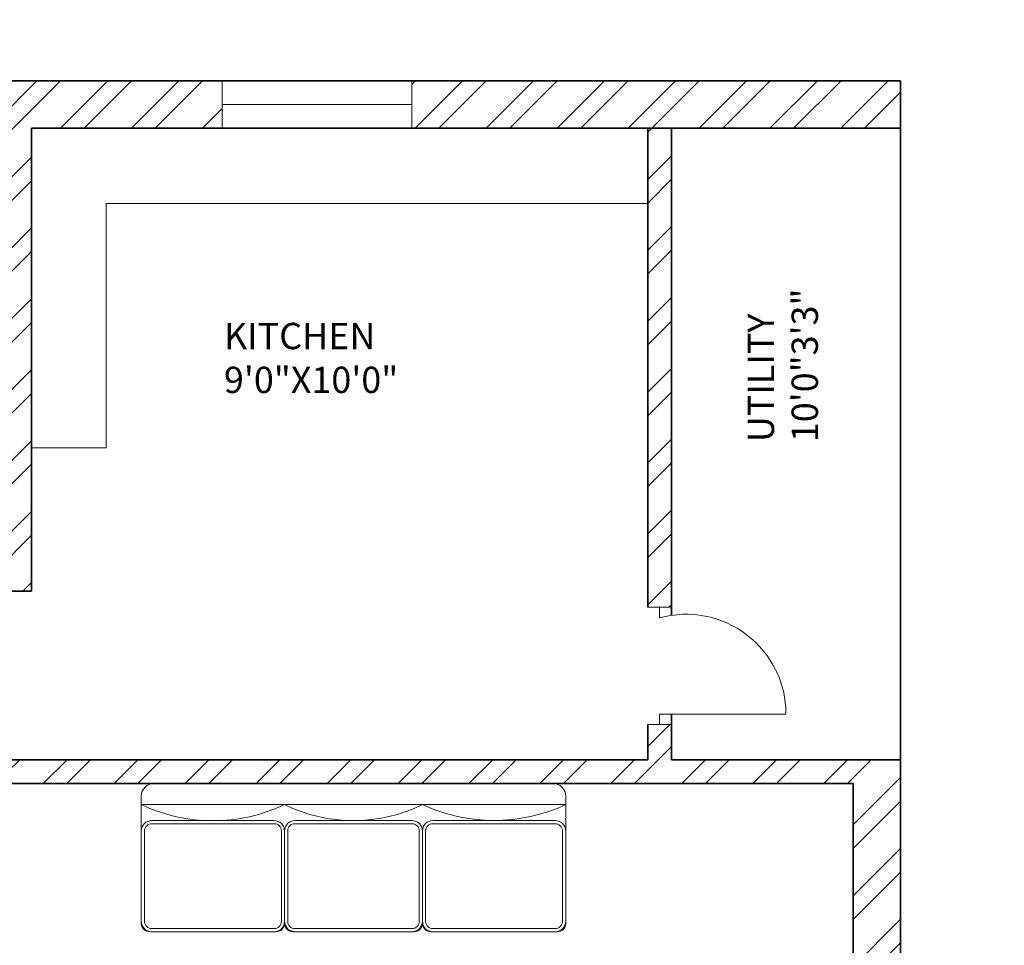
# Model space of a CAD drawing. Units: inches. Extents: x 2120 to 4013, y 1390 to 3019.
# Tile 34 of 59: x 2470 to 2657, y 2188 to 2364. Entities that reach past the tile are written whole.
import ezdxf

# ---------------------------------------------------------------- set-up
doc = ezdxf.new("R2010")
doc.units = ezdxf.units.IN
for name, color, linetype, lineweight in [('A-ANNO-DIMS', 2, 'Continuous', 18), ('A-AREA-IDEN', 7, 'Continuous', 18), ('A-DOOR', 3, 'Continuous', 18), ('A-FLOR-CASE', 8, 'Continuous', 18), ('A-FURN', 8, 'Continuous', 13), ('A-GLAZ', 4, 'Continuous', 18), ('A-WALL', 7, 'Continuous', 35), ('A-WALL-PATT', 252, 'Continuous', 13)]:
    doc.layers.add(name, color=color, linetype=linetype, lineweight=lineweight)
doc.styles.get("Standard").update_dxf_attribs({"font": 'arial.ttf'})
doc.dimstyles.get("Standard").update_dxf_attribs({"dimtxt": 0.18, "dimasz": 0.18, "dimexe": 0.18, "dimexo": 0.0625, "dimgap": 0.09, "dimtad": 0, "dimtih": 1, "dimtoh": 1, "dimdec": 4, "dimzin": 0, "dimdsep": 46, "dimtxsty": 'Standard', "dimcen": 0.09, "dimadec": 0, "dimazin": 0, "dimtfac": 1, "dimtdec": 4, "dimtofl": 0, "dimtmove": 0, "dimatfit": 3, "dimfxl": 1, "dimtolj": 1, "dimtzin": 0, "dimarcsym": 0})

# ---------------------------------------------------------------- blocks, each defined once
blk = doc.blocks.new('DOOR-SWING-24IN-105p37DEG')
for p, q in [((4.5, 22.29), (0, 22.29)), ((0, 22.29), (2.25, 22.29)), ((2.25, 22.29), (2.25, 20.29)), ((2.25, 0), (2.25, 2)), ((2.25, 2), (26.25, 2)), ((0, 0), (4.5, 0)), ((4.5, 0), (2.25, 0))]:
    blk.add_line(p, q)
blk.add_arc((7.28, 2), 18.97, 0, 105.3718)
blk = doc.blocks.new('WIN-PLAN-36IN')
for p, q in [((0, 0), (0, 9)), ((0, 9), (0, 4.5)), ((36, 4.5), (36, 9)), ((36, 9), (36, 0)), ((0, 4.5), (36, 4.5))]:
    blk.add_line(p, q)
blk = doc.blocks.new('*D211')
at = {"layer": 'A-ANNO-DIMS', "color": 0, "lineweight": -2, "transparency": 16777216}
for p, q in [((2262.73, 2352.59), (2262.73, 2397.71)), ((2262.91, 2397.53), (2635.95, 2397.53)), ((3009.55, 2397.53), (2636.52, 2397.53)), ((3009.73, 2352.59), (3009.73, 2397.71))]:
    blk.add_line(p, q, dxfattribs=at)
at = {"layer": 'A-ANNO-DIMS', "color": 0, "transparency": 16777216}
for points in [[(2262.91, 2397.56), (2262.91, 2397.5), (2262.73, 2397.53)], [(3009.55, 2397.56), (3009.55, 2397.5), (3009.73, 2397.53)]]:
    blk.add_solid(points, dxfattribs=at)
at = {"layer": 'Defpoints', "color": 0, "transparency": 16777216}
for p in [(3009.73, 2397.53), (2262.73, 2352.53), (3009.73, 2352.53)]:
    blk.add_point(p, dxfattribs=at)
at = {"layer": 'A-ANNO-DIMS', "color": 0, "transparency": 16777216, "insert": (2636.23, 2397.53), "char_height": 0.18, "attachment_point": 5}
blk.add_mtext('\\A1;747', dxfattribs=at)

msp = doc.modelspace()

# ---------------------------------------------------------------- hatches: boundary and pattern name
at = {"layer": 'A-WALL-PATT'}
h = msp.add_hatch(dxfattribs=at)
h.set_pattern_fill('ANSI32', color=256)
h.paths.add_polyline_path([(2271.7331, 2343.531), (2283.3788, 2343.531), (2283.3788, 2348.031), (2283.3788, 2352.5306), (2262.7331, 2352.5306), (2262.7331, 2182.638), (2267.2331, 2182.638), (2271.7331, 2182.638), (2271.7331, 2219.031), (2391.7331, 2219.031), (2391.7331, 2214.189), (2393.9831, 2214.189), (2396.2331, 2214.189), (2396.2331, 2219.031), (2420.2331, 2219.031), (2420.2331, 2225.7535), (2417.2197, 2225.7535), (2415.7331, 2225.7535), (2415.7331, 2223.5306), (2271.7331, 2223.5306)])
h.paths.add_polyline_path([(2380.0942, 2352.5306), (2343.3788, 2352.5306), (2343.3788, 2343.531), (2363.2331, 2343.531), (2363.2331, 2288.8489), (2365.4831, 2288.8489), (2367.7331, 2288.8489), (2367.7331, 2343.531), (2380.0942, 2343.531)], flags=17)
h.paths.add_polyline_path([(2432.4339, 2352.5306), (2404.0943, 2352.5306), (2404.0943, 2343.531), (2415.7331, 2343.531), (2415.7331, 2264.0306), (2367.7331, 2264.0306), (2367.7331, 2266.4872), (2363.2331, 2266.4872), (2363.2331, 2259.531), (2367.7331, 2259.531), (2415.7331, 2259.531), (2415.7331, 2255.0658), (2420.2331, 2255.0658), (2420.2331, 2259.531), (2424.5717, 2259.531), (2424.5717, 2261.781), (2424.5717, 2264.0306), (2420.2331, 2264.0306), (2420.2331, 2343.531), (2432.4339, 2343.531)])
h.paths.add_polyline_path([(2508.9115, 2352.5306), (2456.4339, 2352.5306), (2456.4339, 2343.531), (2468.2331, 2343.531), (2468.2331, 2264.0306), (2448.0487, 2264.0306), (2448.0487, 2259.531), (2468.2331, 2259.531), (2468.2331, 2255.5496), (2472.7331, 2255.5496), (2472.7331, 2343.531), (2508.9115, 2343.531)])
h.paths.add_polyline_path([(2637.7331, 2352.5306), (2544.9116, 2352.5306), (2544.9116, 2343.531), (2589.7331, 2343.531), (2633.2331, 2343.531), (2637.7331, 2343.531)])
h.paths.add_polyline_path([(2594.2331, 2343.5306), (2589.7331, 2343.5306), (2589.7331, 2259.5306), (2589.7331, 2252.4915), (2591.9831, 2252.4915), (2594.2331, 2252.4915)])
h.paths.add_polyline_path([(2637.7331, 2223.5306), (2594.2331, 2223.5306), (2594.2331, 2230.1988), (2591.9831, 2230.1988), (2589.7331, 2230.1988), (2589.7331, 2223.5306), (2472.7331, 2223.5306), (2468.2331, 2223.5306), (2468.2331, 2219.031), (2628.7331, 2219.031), (2628.7331, 2138.031), (2637.7331, 2138.031)])
h.paths.add_polyline_path([(3822.6535, 2458.4402), (3874.9468, 2458.4402), (3874.9468, 2476.9866), (3822.6535, 2476.9866)], flags=9)
h.paths.add_polyline_path([(3834.6921, 2781.8174), (3935.9206, 2781.8174), (3935.9206, 2800.3638), (3834.6921, 2800.3638)], flags=9)
h.paths.add_polyline_path([(3832.2843, 2837.9683), (3884.5776, 2837.9683), (3884.5776, 2856.5146), (3832.2843, 2856.5146)], flags=9)
h.paths.add_polyline_path([(3830.9388, 2861.4782), (3956.8958, 2861.4782), (3956.8958, 2880.0245), (3830.9388, 2880.0245)], flags=9)
h.paths.add_polyline_path([(3870.6966, 2352.5752), (3887.9272, 2352.5752), (3887.9272, 2377.3037), (3870.6966, 2377.3037)], flags=9)
h.paths.add_polyline_path([(3289.2701, 2413.161), (3435.2223, 2413.161), (3435.2223, 2450.2538), (3289.2701, 2450.2538)], flags=9)
h.paths.add_polyline_path([(2487.6944, 2414.3601), (2637.8335, 2414.3601), (2637.8335, 2451.4528), (2487.6944, 2451.4528)], flags=9)
h.paths.add_polyline_path([(2567.3724, 1457.9199), (2815.296, 1457.9199), (2815.296, 1495.0127), (2567.3724, 1495.0127)], flags=9)
h.paths.add_polyline_path([(2655.3825, 2093.2363), (2685.9555, 2093.2363), (2685.9555, 2111.8937), (2655.3825, 2111.8937)], flags=9)
h.paths.add_polyline_path([(2543.9218, 1550.6671), (2587.8406, 1550.6671), (2587.8406, 1569.3244), (2543.9218, 1569.3244)], flags=9)
h.paths.add_polyline_path([(2905.1384, 1543.8113), (2949.0572, 1543.8113), (2949.0572, 1562.4686), (2905.1384, 1562.4686)], flags=9)
h.paths.add_polyline_path([(2736.4118, 1702.4736), (2784.2153, 1702.4736), (2784.2153, 1721.1309), (2736.4118, 1721.1309)], flags=9)
h.paths.add_polyline_path([(2912.8666, 1710.4168), (2951.707, 1710.4168), (2951.707, 1729.0741), (2912.8666, 1729.0741)], flags=9)
h.paths.add_polyline_path([(2923.5785, 1763.5038), (2959.7279, 1763.5038), (2959.7279, 1782.1611), (2923.5785, 1782.1611)], flags=9)
h.paths.add_polyline_path([(2925.2114, 1809.6137), (2967.1861, 1809.6137), (2967.1861, 1828.271), (2925.2114, 1828.271)], flags=9)
h.paths.add_polyline_path([(2996.2711, 1878.9003), (2996.2711, 1913.109), (2977.6138, 1913.109), (2977.6138, 1878.9003)], flags=9)
h.paths.add_polyline_path([(2883.0859, 1895.7192), (2927.1855, 1895.7192), (2927.1855, 1914.3766), (2883.0859, 1914.3766)], flags=9)
h.paths.add_polyline_path([(2787.3924, 1810.8013), (2841.0213, 1810.8013), (2841.0213, 1829.4587), (2787.3924, 1829.4587)], flags=9)
h.paths.add_polyline_path([(2775.6399, 2101.7395), (2829.2689, 2101.7395), (2829.2689, 2120.3968), (2775.6399, 2120.3968)], flags=9)
h.paths.add_polyline_path([(2913.0263, 2075.817), (2951.8667, 2075.817), (2951.8667, 2094.4744), (2913.0263, 2094.4744)], flags=9)
h.paths.add_polyline_path([(2929.966, 2133.3669), (2966.1154, 2133.3669), (2966.1154, 2152.0243), (2929.966, 2152.0243)], flags=9)
h.paths.add_polyline_path([(2932.7502, 2182.6088), (2968.8996, 2182.6088), (2968.8996, 2201.2662), (2932.7502, 2201.2662)], flags=9)
h.paths.add_polyline_path([(2996.0681, 2266.3173), (2996.0681, 2300.5261), (2977.4108, 2300.5261), (2977.4108, 2266.3173)], flags=9)
h.paths.add_polyline_path([(2885.1039, 2279.2186), (2929.2035, 2279.2186), (2929.2035, 2297.8759), (2885.1039, 2297.8759)], flags=9)
h.paths.add_polyline_path([(2735.7042, 2218.3197), (2783.5078, 2218.3197), (2783.5078, 2236.9771), (2735.7042, 2236.9771)], flags=9)
h.paths.add_polyline_path([(2635.6049, 2044.0085), (2648.9678, 2044.0085), (2648.9678, 2054.312), (2635.6049, 2054.312)], flags=9)
h.paths.add_polyline_path([(2714.0148, 1923.0473), (2727.3777, 1923.0473), (2727.3777, 1933.3508), (2714.0148, 1933.3508)], flags=9)
h.paths.add_polyline_path([(2709.0345, 1988.1628), (2722.3974, 1988.1628), (2722.3974, 1998.4663), (2709.0345, 1998.4663)], flags=9)
h.paths.add_polyline_path([(2592.8935, 1962.1763), (2606.2564, 1962.1763), (2606.2564, 1972.4799), (2592.8935, 1972.4799)], flags=9)
h.paths.add_polyline_path([(2618.3996, 1985.9724), (2644.1942, 1985.9724), (2644.1942, 1996.2759), (2618.3996, 1996.2759)], flags=9)
h.paths.add_polyline_path([(2601.279, 1920.5869), (2614.6419, 1920.5869), (2614.6419, 1930.8904), (2601.279, 1930.8904)], flags=9)
h.paths.add_polyline_path([(2692.3278, 1932.7645), (2704.5311, 1932.7645), (2704.5311, 1943.0681), (2692.3278, 1943.0681)], flags=9)
h.paths.add_polyline_path([(2311.122, 1672.7318), (2355.0408, 1672.7318), (2355.0408, 1691.3892), (2311.122, 1691.3892)], flags=9)
h.paths.add_polyline_path([(2456.2551, 1632.3198), (2492.4796, 1632.3198), (2492.4796, 1650.9772), (2456.2551, 1650.9772)], flags=9)
h.paths.add_polyline_path([(2401.0766, 1631.4793), (2437.301, 1631.4793), (2437.301, 1650.1367), (2401.0766, 1650.1367)], flags=9)
h.paths.add_polyline_path([(2546.7054, 1700.9235), (2594.509, 1700.9235), (2594.509, 1719.5809), (2546.7054, 1719.5809)], flags=9)
h.paths.add_polyline_path([(2445.4866, 1766.9937), (2497.5261, 1766.9937), (2497.5261, 1785.651), (2445.4866, 1785.651)], flags=9)
h.paths.add_polyline_path([(2287.9992, 1739.7675), (2326.8396, 1739.7675), (2326.8396, 1758.4248), (2287.9992, 1758.4248)], flags=9)
h.paths.add_polyline_path([(2458.5279, 1924.7607), (2510.5675, 1924.7607), (2510.5675, 1943.4181), (2458.5279, 1943.4181)], flags=9)
h.paths.add_polyline_path([(2309.2811, 1902.7642), (2345.4305, 1902.7642), (2345.4305, 1921.4215), (2309.2811, 1921.4215)], flags=9)
h.paths.add_polyline_path([(2490.7554, 2018.9392), (2530.7896, 2018.9392), (2530.7896, 2037.5965), (2490.7554, 2037.5965)], flags=9)
h.paths.add_polyline_path([(2402.143, 2024.7393), (2438.5414, 2024.7393), (2438.5414, 2043.3966), (2402.143, 2043.3966)], flags=9)
h.paths.add_polyline_path([(2287.856, 1931.7926), (2326.6964, 1931.7926), (2326.6964, 1950.4499), (2287.856, 1950.4499)], flags=9)
h.paths.add_polyline_path([(2281.7979, 2193.5771), (2320.6383, 2193.5771), (2320.6383, 2212.2344), (2281.7979, 2212.2344)], flags=25)
h.paths.add_polyline_path([(2484.0754, 2093.892), (2536.115, 2093.892), (2536.115, 2112.5494), (2484.0754, 2112.5494)], flags=9)
h.paths.add_polyline_path([(2624.7948, 2281.8639), (2624.7948, 2311.4137), (2606.1375, 2311.4137), (2606.1375, 2281.8639)], flags=9)
h.paths.add_polyline_path([(2507.5036, 2290.3639), (2541.934, 2290.3639), (2541.934, 2309.0212), (2507.5036, 2309.0212)], flags=9)
h.paths.add_polyline_path([(2423.1076, 2285.2202), (2459.332, 2285.2202), (2459.332, 2303.8776), (2423.1076, 2303.8776)], flags=9)
h.paths.add_polyline_path([(2374.5467, 2289.6272), (2410.7711, 2289.6272), (2410.7711, 2308.2846), (2374.5467, 2308.2846)], flags=25)
h.paths.add_polyline_path([(2277.4907, 2227.5651), (2316.3311, 2227.5651), (2316.3311, 2246.2224), (2277.4907, 2246.2224)], flags=25)
h.paths.add_polyline_path([(2655.3825, 2093.2367), (2685.9555, 2093.2367), (2685.9555, 2111.894), (2655.3825, 2111.894)], flags=9)
h.paths.add_polyline_path([(2543.9217, 1550.6674), (2587.8406, 1550.6674), (2587.8406, 1569.3247), (2543.9217, 1569.3247)], flags=9)
h.paths.add_polyline_path([(2905.1384, 1543.8116), (2949.0572, 1543.8116), (2949.0572, 1562.4689), (2905.1384, 1562.4689)], flags=9)
h.paths.add_polyline_path([(2736.4118, 1702.4739), (2784.2153, 1702.4739), (2784.2153, 1721.1312), (2736.4118, 1721.1312)], flags=9)
h.paths.add_polyline_path([(2912.8666, 1710.4171), (2951.707, 1710.4171), (2951.707, 1729.0744), (2912.8666, 1729.0744)], flags=9)
h.paths.add_polyline_path([(2923.5785, 1763.5041), (2959.7279, 1763.5041), (2959.7279, 1782.1614), (2923.5785, 1782.1614)], flags=9)
h.paths.add_polyline_path([(2925.2114, 1809.614), (2967.1861, 1809.614), (2967.1861, 1828.2713), (2925.2114, 1828.2713)], flags=9)
h.paths.add_polyline_path([(2996.2711, 1878.9006), (2996.2711, 1913.1094), (2977.6137, 1913.1094), (2977.6137, 1878.9006)], flags=9)
h.paths.add_polyline_path([(2883.0859, 1895.7195), (2927.1855, 1895.7195), (2927.1855, 1914.3769), (2883.0859, 1914.3769)], flags=9)
h.paths.add_polyline_path([(2787.3924, 1810.8016), (2841.0213, 1810.8016), (2841.0213, 1829.459), (2787.3924, 1829.459)], flags=9)
h.paths.add_polyline_path([(2775.6399, 2101.7398), (2829.2688, 2101.7398), (2829.2688, 2120.3971), (2775.6399, 2120.3971)], flags=9)
h.paths.add_polyline_path([(2913.0263, 2075.8173), (2951.8667, 2075.8173), (2951.8667, 2094.4747), (2913.0263, 2094.4747)], flags=9)
h.paths.add_polyline_path([(2929.966, 2133.3672), (2966.1154, 2133.3672), (2966.1154, 2152.0246), (2929.966, 2152.0246)], flags=9)
h.paths.add_polyline_path([(2932.7502, 2182.6091), (2968.8996, 2182.6091), (2968.8996, 2201.2665), (2932.7502, 2201.2665)], flags=9)
h.paths.add_polyline_path([(2996.0681, 2266.3176), (2996.0681, 2300.5264), (2977.4108, 2300.5264), (2977.4108, 2266.3176)], flags=9)
h.paths.add_polyline_path([(2885.1039, 2279.2189), (2929.2035, 2279.2189), (2929.2035, 2297.8762), (2885.1039, 2297.8762)], flags=9)
h.paths.add_polyline_path([(2735.7042, 2218.32), (2783.5078, 2218.32), (2783.5078, 2236.9774), (2735.7042, 2236.9774)], flags=9)
h.paths.add_polyline_path([(2635.6048, 2044.0088), (2648.9677, 2044.0088), (2648.9677, 2054.3123), (2635.6048, 2054.3123)], flags=9)
h.paths.add_polyline_path([(2714.0148, 1923.0476), (2727.3777, 1923.0476), (2727.3777, 1933.3511), (2714.0148, 1933.3511)], flags=9)
h.paths.add_polyline_path([(2709.0345, 1988.1631), (2722.3974, 1988.1631), (2722.3974, 1998.4666), (2709.0345, 1998.4666)], flags=9)
h.paths.add_polyline_path([(2592.8935, 1962.1766), (2606.2564, 1962.1766), (2606.2564, 1972.4802), (2592.8935, 1972.4802)], flags=9)
h.paths.add_polyline_path([(2618.3995, 1985.9727), (2644.1942, 1985.9727), (2644.1942, 1996.2762), (2618.3995, 1996.2762)], flags=9)
h.paths.add_polyline_path([(2601.279, 1920.5872), (2614.6419, 1920.5872), (2614.6419, 1930.8908), (2601.279, 1930.8908)], flags=9)
h.paths.add_polyline_path([(2692.3278, 1932.7648), (2704.5311, 1932.7648), (2704.5311, 1943.0684), (2692.3278, 1943.0684)], flags=9)
h.paths.add_polyline_path([(2311.122, 1672.7321), (2355.0408, 1672.7321), (2355.0408, 1691.3895), (2311.122, 1691.3895)], flags=9)
h.paths.add_polyline_path([(2456.2551, 1632.3201), (2492.4795, 1632.3201), (2492.4795, 1650.9775), (2456.2551, 1650.9775)], flags=9)
h.paths.add_polyline_path([(2401.0766, 1631.4796), (2437.301, 1631.4796), (2437.301, 1650.137), (2401.0766, 1650.137)], flags=9)
h.paths.add_polyline_path([(2546.7054, 1700.9238), (2594.509, 1700.9238), (2594.509, 1719.5812), (2546.7054, 1719.5812)], flags=9)
h.paths.add_polyline_path([(2445.4866, 1766.994), (2497.5261, 1766.994), (2497.5261, 1785.6513), (2445.4866, 1785.6513)], flags=9)
h.paths.add_polyline_path([(2287.9992, 1739.7678), (2326.8396, 1739.7678), (2326.8396, 1758.4251), (2287.9992, 1758.4251)], flags=9)
h.paths.add_polyline_path([(2458.5279, 1924.7611), (2510.5675, 1924.7611), (2510.5675, 1943.4184), (2458.5279, 1943.4184)], flags=9)
h.paths.add_polyline_path([(2309.2811, 1902.7645), (2345.4305, 1902.7645), (2345.4305, 1921.4218), (2309.2811, 1921.4218)], flags=9)
h.paths.add_polyline_path([(2490.7554, 2018.9395), (2530.7895, 2018.9395), (2530.7895, 2037.5968), (2490.7554, 2037.5968)], flags=9)
h.paths.add_polyline_path([(2402.143, 2024.7396), (2438.5413, 2024.7396), (2438.5413, 2043.3969), (2402.143, 2043.3969)], flags=9)
h.paths.add_polyline_path([(2287.856, 1931.7929), (2326.6964, 1931.7929), (2326.6964, 1950.4502), (2287.856, 1950.4502)], flags=9)
h.paths.add_polyline_path([(2281.7979, 2193.5774), (2320.6383, 2193.5774), (2320.6383, 2212.2347), (2281.7979, 2212.2347)], flags=25)
h.paths.add_polyline_path([(2484.0754, 2093.8924), (2536.115, 2093.8924), (2536.115, 2112.5497), (2484.0754, 2112.5497)], flags=9)
h.paths.add_polyline_path([(2624.7948, 2281.8642), (2624.7948, 2311.414), (2606.1374, 2311.414), (2606.1374, 2281.8642)], flags=9)
h.paths.add_polyline_path([(2507.5035, 2290.3642), (2541.934, 2290.3642), (2541.934, 2309.0215), (2507.5035, 2309.0215)], flags=9)
h.paths.add_polyline_path([(2423.1075, 2285.2205), (2459.332, 2285.2205), (2459.332, 2303.8779), (2423.1075, 2303.8779)], flags=9)
h.paths.add_polyline_path([(2374.5467, 2289.6275), (2410.7711, 2289.6275), (2410.7711, 2308.2849), (2374.5467, 2308.2849)], flags=25)
h.paths.add_polyline_path([(2277.4907, 2227.5654), (2316.3311, 2227.5654), (2316.3311, 2246.2227), (2277.4907, 2246.2227)], flags=25)
h = msp.add_hatch(dxfattribs=at)
h.set_pattern_fill('ANSI32', color=256)
h.paths.add_polyline_path([(2271.7331, 1980.389), (2262.7331, 1980.389), (2262.7331, 1912.8434), (2267.2331, 1912.8434), (2271.7331, 1912.8434), (2271.7331, 1922.531), (2351.2331, 1922.531), (2351.2331, 1901.4728), (2355.7331, 1901.4728), (2355.7331, 1922.531), (2357.9815, 1922.531), (2357.9815, 1926.5306), (2271.7331, 1926.5306)])
h.paths.add_polyline_path([(2589.2331, 1949.1622), (2584.7331, 1949.1622), (2580.2331, 1949.1622), (2580.2331, 1874.5306), (2355.7331, 1874.5306), (2355.7331, 1880.1922), (2351.2331, 1880.1922), (2351.2331, 1874.5306), (2271.7331, 1874.5306), (2271.7331, 1888.8431), (2262.7331, 1888.8431), (2262.7331, 1842.2909), (2267.2331, 1842.2909), (2271.7331, 1842.2909), (2271.7331, 1865.531), (2415.7331, 1865.531), (2415.7331, 1779.7286), (2420.2331, 1779.7286), (2420.2331, 1865.531), (2589.2331, 1865.531)])
h.paths.add_polyline_path([(2271.7331, 1782.2906), (2262.7331, 1782.2906), (2262.7331, 1711.4639), (2267.2331, 1711.4639), (2271.7331, 1711.4639), (2271.7331, 1738.031), (2420.2331, 1738.031), (2420.2331, 1742.531), (2420.2331, 1747.3376), (2417.9831, 1747.3376), (2415.7331, 1747.3376), (2415.7331, 1742.5306), (2271.7331, 1742.5306)])
h.paths.add_polyline_path([(2271.7331, 1627.031), (2362.3957, 1627.031), (2362.3957, 1629.281), (2362.3957, 1631.5306), (2271.7331, 1631.5306), (2271.7331, 1675.4636), (2262.7331, 1675.4636), (2262.7331, 1581.531), (2405.3032, 1581.531), (2405.3032, 1586.031), (2405.3032, 1590.5306), (2396.2331, 1590.5306), (2396.2331, 1691.4513), (2418.7206, 1691.4513), (2418.7206, 1695.951), (2396.2331, 1695.951), (2391.7331, 1695.951), (2391.7331, 1631.5306), (2386.7425, 1631.5306), (2386.7425, 1629.2806), (2386.7425, 1627.031), (2391.7331, 1627.031), (2391.7331, 1586.1709), (2271.7331, 1586.1709)])
h.paths.add_polyline_path([(2459.6703, 1590.5306), (2429.3032, 1590.5306), (2429.3032, 1581.531), (2459.6703, 1581.531), (2459.6703, 1586.031)])
h.paths.add_polyline_path([(2501.2331, 1590.531), (2501.2331, 1665.0195), (2498.9831, 1665.0195), (2496.7331, 1665.0195), (2496.7331, 1590.5306), (2483.8201, 1590.5306), (2483.8201, 1590.1579), (2483.6704, 1590.1579), (2483.6704, 1581.531), (2505.0196, 1581.531), (2505.0196, 1583.781), (2505.0196, 1586.0306), (2501.2331, 1586.0306)])
h.paths.add_polyline_path([(2544.1361, 1583.781), (2544.1361, 1586.0306), (2527.1368, 1586.0306), (2527.1368, 1583.7806), (2527.1368, 1581.531), (2544.1361, 1581.531)])
h.paths.add_polyline_path([(3822.6535, 2458.4402), (3874.9468, 2458.4402), (3874.9468, 2476.9866), (3822.6535, 2476.9866)], flags=9)
h.paths.add_polyline_path([(3834.6921, 2781.8174), (3935.9206, 2781.8174), (3935.9206, 2800.3638), (3834.6921, 2800.3638)], flags=9)
h.paths.add_polyline_path([(3832.2843, 2837.9683), (3884.5776, 2837.9683), (3884.5776, 2856.5146), (3832.2843, 2856.5146)], flags=9)
h.paths.add_polyline_path([(3830.9388, 2861.4782), (3956.8958, 2861.4782), (3956.8958, 2880.0245), (3830.9388, 2880.0245)], flags=9)
h.paths.add_polyline_path([(3870.6966, 2352.5752), (3887.9272, 2352.5752), (3887.9272, 2377.3037), (3870.6966, 2377.3037)], flags=9)
h.paths.add_polyline_path([(3289.2701, 2413.161), (3435.2223, 2413.161), (3435.2223, 2450.2538), (3289.2701, 2450.2538)], flags=9)
h.paths.add_polyline_path([(2487.6944, 2414.3601), (2637.8335, 2414.3601), (2637.8335, 2451.4528), (2487.6944, 2451.4528)], flags=9)
h.paths.add_polyline_path([(2567.3724, 1457.9199), (2815.296, 1457.9199), (2815.296, 1495.0127), (2567.3724, 1495.0127)], flags=9)
h.paths.add_polyline_path([(2655.3825, 2093.2363), (2685.9555, 2093.2363), (2685.9555, 2111.8937), (2655.3825, 2111.8937)], flags=9)
h.paths.add_polyline_path([(2543.9218, 1550.6671), (2587.8406, 1550.6671), (2587.8406, 1569.3244), (2543.9218, 1569.3244)], flags=9)
h.paths.add_polyline_path([(2905.1384, 1543.8113), (2949.0572, 1543.8113), (2949.0572, 1562.4686), (2905.1384, 1562.4686)], flags=9)
h.paths.add_polyline_path([(2736.4118, 1702.4736), (2784.2153, 1702.4736), (2784.2153, 1721.1309), (2736.4118, 1721.1309)], flags=9)
h.paths.add_polyline_path([(2912.8666, 1710.4168), (2951.707, 1710.4168), (2951.707, 1729.0741), (2912.8666, 1729.0741)], flags=9)
h.paths.add_polyline_path([(2923.5785, 1763.5038), (2959.7279, 1763.5038), (2959.7279, 1782.1611), (2923.5785, 1782.1611)], flags=9)
h.paths.add_polyline_path([(2925.2114, 1809.6137), (2967.1861, 1809.6137), (2967.1861, 1828.271), (2925.2114, 1828.271)], flags=9)
h.paths.add_polyline_path([(2996.2711, 1878.9003), (2996.2711, 1913.109), (2977.6138, 1913.109), (2977.6138, 1878.9003)], flags=9)
h.paths.add_polyline_path([(2883.0859, 1895.7192), (2927.1855, 1895.7192), (2927.1855, 1914.3766), (2883.0859, 1914.3766)], flags=9)
h.paths.add_polyline_path([(2787.3924, 1810.8013), (2841.0213, 1810.8013), (2841.0213, 1829.4587), (2787.3924, 1829.4587)], flags=9)
h.paths.add_polyline_path([(2775.6399, 2101.7395), (2829.2689, 2101.7395), (2829.2689, 2120.3968), (2775.6399, 2120.3968)], flags=9)
h.paths.add_polyline_path([(2913.0263, 2075.817), (2951.8667, 2075.817), (2951.8667, 2094.4744), (2913.0263, 2094.4744)], flags=9)
h.paths.add_polyline_path([(2929.966, 2133.3669), (2966.1154, 2133.3669), (2966.1154, 2152.0243), (2929.966, 2152.0243)], flags=9)
h.paths.add_polyline_path([(2932.7502, 2182.6088), (2968.8996, 2182.6088), (2968.8996, 2201.2662), (2932.7502, 2201.2662)], flags=9)
h.paths.add_polyline_path([(2996.0681, 2266.3173), (2996.0681, 2300.5261), (2977.4108, 2300.5261), (2977.4108, 2266.3173)], flags=9)
h.paths.add_polyline_path([(2885.1039, 2279.2186), (2929.2035, 2279.2186), (2929.2035, 2297.8759), (2885.1039, 2297.8759)], flags=9)
h.paths.add_polyline_path([(2735.7042, 2218.3197), (2783.5078, 2218.3197), (2783.5078, 2236.9771), (2735.7042, 2236.9771)], flags=9)
h.paths.add_polyline_path([(2635.6049, 2044.0085), (2648.9678, 2044.0085), (2648.9678, 2054.312), (2635.6049, 2054.312)], flags=9)
h.paths.add_polyline_path([(2714.0148, 1923.0473), (2727.3777, 1923.0473), (2727.3777, 1933.3508), (2714.0148, 1933.3508)], flags=9)
h.paths.add_polyline_path([(2709.0345, 1988.1628), (2722.3974, 1988.1628), (2722.3974, 1998.4663), (2709.0345, 1998.4663)], flags=9)
h.paths.add_polyline_path([(2592.8935, 1962.1763), (2606.2564, 1962.1763), (2606.2564, 1972.4799), (2592.8935, 1972.4799)], flags=9)
h.paths.add_polyline_path([(2618.3996, 1985.9724), (2644.1942, 1985.9724), (2644.1942, 1996.2759), (2618.3996, 1996.2759)], flags=9)
h.paths.add_polyline_path([(2601.279, 1920.5869), (2614.6419, 1920.5869), (2614.6419, 1930.8904), (2601.279, 1930.8904)], flags=9)
h.paths.add_polyline_path([(2692.3278, 1932.7645), (2704.5311, 1932.7645), (2704.5311, 1943.0681), (2692.3278, 1943.0681)], flags=9)
h.paths.add_polyline_path([(2311.122, 1672.7318), (2355.0408, 1672.7318), (2355.0408, 1691.3892), (2311.122, 1691.3892)], flags=25)
h.paths.add_polyline_path([(2456.2551, 1632.3198), (2492.4796, 1632.3198), (2492.4796, 1650.9772), (2456.2551, 1650.9772)], flags=9)
h.paths.add_polyline_path([(2401.0766, 1631.4793), (2437.301, 1631.4793), (2437.301, 1650.1367), (2401.0766, 1650.1367)], flags=9)
h.paths.add_polyline_path([(2546.7054, 1700.9235), (2594.509, 1700.9235), (2594.509, 1719.5809), (2546.7054, 1719.5809)], flags=9)
h.paths.add_polyline_path([(2445.4866, 1766.9937), (2497.5261, 1766.9937), (2497.5261, 1785.651), (2445.4866, 1785.651)], flags=9)
h.paths.add_polyline_path([(2287.9992, 1739.7675), (2326.8396, 1739.7675), (2326.8396, 1758.4248), (2287.9992, 1758.4248)], flags=24)
h.paths.add_polyline_path([(2458.5279, 1924.7607), (2510.5675, 1924.7607), (2510.5675, 1943.4181), (2458.5279, 1943.4181)], flags=25)
h.paths.add_polyline_path([(2309.2811, 1902.7642), (2345.4305, 1902.7642), (2345.4305, 1921.4215), (2309.2811, 1921.4215)], flags=25)
h.paths.add_polyline_path([(2490.7554, 2018.9392), (2530.7896, 2018.9392), (2530.7896, 2037.5965), (2490.7554, 2037.5965)], flags=9)
h.paths.add_polyline_path([(2402.143, 2024.7393), (2438.5414, 2024.7393), (2438.5414, 2043.3966), (2402.143, 2043.3966)], flags=9)
h.paths.add_polyline_path([(2287.856, 1931.7926), (2326.6964, 1931.7926), (2326.6964, 1950.4499), (2287.856, 1950.4499)], flags=25)
h.paths.add_polyline_path([(2281.7979, 2193.5771), (2320.6383, 2193.5771), (2320.6383, 2212.2344), (2281.7979, 2212.2344)], flags=9)
h.paths.add_polyline_path([(2484.0754, 2093.892), (2536.115, 2093.892), (2536.115, 2112.5494), (2484.0754, 2112.5494)], flags=9)
h.paths.add_polyline_path([(2624.7948, 2281.8639), (2624.7948, 2311.4137), (2606.1375, 2311.4137), (2606.1375, 2281.8639)], flags=9)
h.paths.add_polyline_path([(2507.5036, 2290.3639), (2541.934, 2290.3639), (2541.934, 2309.0212), (2507.5036, 2309.0212)], flags=9)
h.paths.add_polyline_path([(2423.1076, 2285.2202), (2459.332, 2285.2202), (2459.332, 2303.8776), (2423.1076, 2303.8776)], flags=9)
h.paths.add_polyline_path([(2374.5467, 2289.6272), (2410.7711, 2289.6272), (2410.7711, 2308.2846), (2374.5467, 2308.2846)], flags=9)
h.paths.add_polyline_path([(2277.4907, 2227.5651), (2316.3311, 2227.5651), (2316.3311, 2246.2224), (2277.4907, 2246.2224)], flags=9)
h.paths.add_polyline_path([(2655.3825, 2093.2367), (2685.9555, 2093.2367), (2685.9555, 2111.894), (2655.3825, 2111.894)], flags=9)
h.paths.add_polyline_path([(2543.9217, 1550.6674), (2587.8406, 1550.6674), (2587.8406, 1569.3247), (2543.9217, 1569.3247)], flags=9)
h.paths.add_polyline_path([(2905.1384, 1543.8116), (2949.0572, 1543.8116), (2949.0572, 1562.4689), (2905.1384, 1562.4689)], flags=9)
h.paths.add_polyline_path([(2736.4118, 1702.4739), (2784.2153, 1702.4739), (2784.2153, 1721.1312), (2736.4118, 1721.1312)], flags=9)
h.paths.add_polyline_path([(2912.8666, 1710.4171), (2951.707, 1710.4171), (2951.707, 1729.0744), (2912.8666, 1729.0744)], flags=9)
h.paths.add_polyline_path([(2923.5785, 1763.5041), (2959.7279, 1763.5041), (2959.7279, 1782.1614), (2923.5785, 1782.1614)], flags=9)
h.paths.add_polyline_path([(2925.2114, 1809.614), (2967.1861, 1809.614), (2967.1861, 1828.2713), (2925.2114, 1828.2713)], flags=9)
h.paths.add_polyline_path([(2996.2711, 1878.9006), (2996.2711, 1913.1094), (2977.6137, 1913.1094), (2977.6137, 1878.9006)], flags=9)
h.paths.add_polyline_path([(2883.0859, 1895.7195), (2927.1855, 1895.7195), (2927.1855, 1914.3769), (2883.0859, 1914.3769)], flags=9)
h.paths.add_polyline_path([(2787.3924, 1810.8016), (2841.0213, 1810.8016), (2841.0213, 1829.459), (2787.3924, 1829.459)], flags=9)
h.paths.add_polyline_path([(2775.6399, 2101.7398), (2829.2688, 2101.7398), (2829.2688, 2120.3971), (2775.6399, 2120.3971)], flags=9)
h.paths.add_polyline_path([(2913.0263, 2075.8173), (2951.8667, 2075.8173), (2951.8667, 2094.4747), (2913.0263, 2094.4747)], flags=9)
h.paths.add_polyline_path([(2929.966, 2133.3672), (2966.1154, 2133.3672), (2966.1154, 2152.0246), (2929.966, 2152.0246)], flags=9)
h.paths.add_polyline_path([(2932.7502, 2182.6091), (2968.8996, 2182.6091), (2968.8996, 2201.2665), (2932.7502, 2201.2665)], flags=9)
h.paths.add_polyline_path([(2996.0681, 2266.3176), (2996.0681, 2300.5264), (2977.4108, 2300.5264), (2977.4108, 2266.3176)], flags=9)
h.paths.add_polyline_path([(2885.1039, 2279.2189), (2929.2035, 2279.2189), (2929.2035, 2297.8762), (2885.1039, 2297.8762)], flags=9)
h.paths.add_polyline_path([(2735.7042, 2218.32), (2783.5078, 2218.32), (2783.5078, 2236.9774), (2735.7042, 2236.9774)], flags=9)
h.paths.add_polyline_path([(2635.6048, 2044.0088), (2648.9677, 2044.0088), (2648.9677, 2054.3123), (2635.6048, 2054.3123)], flags=9)
h.paths.add_polyline_path([(2714.0148, 1923.0476), (2727.3777, 1923.0476), (2727.3777, 1933.3511), (2714.0148, 1933.3511)], flags=9)
h.paths.add_polyline_path([(2709.0345, 1988.1631), (2722.3974, 1988.1631), (2722.3974, 1998.4666), (2709.0345, 1998.4666)], flags=9)
h.paths.add_polyline_path([(2592.8935, 1962.1766), (2606.2564, 1962.1766), (2606.2564, 1972.4802), (2592.8935, 1972.4802)], flags=9)
h.paths.add_polyline_path([(2618.3995, 1985.9727), (2644.1942, 1985.9727), (2644.1942, 1996.2762), (2618.3995, 1996.2762)], flags=9)
h.paths.add_polyline_path([(2601.279, 1920.5872), (2614.6419, 1920.5872), (2614.6419, 1930.8908), (2601.279, 1930.8908)], flags=9)
h.paths.add_polyline_path([(2692.3278, 1932.7648), (2704.5311, 1932.7648), (2704.5311, 1943.0684), (2692.3278, 1943.0684)], flags=9)
h.paths.add_polyline_path([(2311.122, 1672.7321), (2355.0408, 1672.7321), (2355.0408, 1691.3895), (2311.122, 1691.3895)], flags=25)
h.paths.add_polyline_path([(2456.2551, 1632.3201), (2492.4795, 1632.3201), (2492.4795, 1650.9775), (2456.2551, 1650.9775)], flags=9)
h.paths.add_polyline_path([(2401.0766, 1631.4796), (2437.301, 1631.4796), (2437.301, 1650.137), (2401.0766, 1650.137)], flags=9)
h.paths.add_polyline_path([(2546.7054, 1700.9238), (2594.509, 1700.9238), (2594.509, 1719.5812), (2546.7054, 1719.5812)], flags=9)
h.paths.add_polyline_path([(2445.4866, 1766.994), (2497.5261, 1766.994), (2497.5261, 1785.6513), (2445.4866, 1785.6513)], flags=9)
h.paths.add_polyline_path([(2287.9992, 1739.7678), (2326.8396, 1739.7678), (2326.8396, 1758.4251), (2287.9992, 1758.4251)], flags=24)
h.paths.add_polyline_path([(2458.5279, 1924.7611), (2510.5675, 1924.7611), (2510.5675, 1943.4184), (2458.5279, 1943.4184)], flags=25)
h.paths.add_polyline_path([(2309.2811, 1902.7645), (2345.4305, 1902.7645), (2345.4305, 1921.4218), (2309.2811, 1921.4218)], flags=25)
h.paths.add_polyline_path([(2490.7554, 2018.9395), (2530.7895, 2018.9395), (2530.7895, 2037.5968), (2490.7554, 2037.5968)], flags=9)
h.paths.add_polyline_path([(2402.143, 2024.7396), (2438.5413, 2024.7396), (2438.5413, 2043.3969), (2402.143, 2043.3969)], flags=9)
h.paths.add_polyline_path([(2287.856, 1931.7929), (2326.6964, 1931.7929), (2326.6964, 1950.4502), (2287.856, 1950.4502)], flags=25)
h.paths.add_polyline_path([(2281.7979, 2193.5774), (2320.6383, 2193.5774), (2320.6383, 2212.2347), (2281.7979, 2212.2347)], flags=9)
h.paths.add_polyline_path([(2484.0754, 2093.8924), (2536.115, 2093.8924), (2536.115, 2112.5497), (2484.0754, 2112.5497)], flags=9)
h.paths.add_polyline_path([(2624.7948, 2281.8642), (2624.7948, 2311.414), (2606.1374, 2311.414), (2606.1374, 2281.8642)], flags=9)
h.paths.add_polyline_path([(2507.5035, 2290.3642), (2541.934, 2290.3642), (2541.934, 2309.0215), (2507.5035, 2309.0215)], flags=9)
h.paths.add_polyline_path([(2423.1075, 2285.2205), (2459.332, 2285.2205), (2459.332, 2303.8779), (2423.1075, 2303.8779)], flags=9)
h.paths.add_polyline_path([(2374.5467, 2289.6275), (2410.7711, 2289.6275), (2410.7711, 2308.2849), (2374.5467, 2308.2849)], flags=9)
h.paths.add_polyline_path([(2277.4907, 2227.5654), (2316.3311, 2227.5654), (2316.3311, 2246.2227), (2277.4907, 2246.2227)], flags=9)

# ---------------------------------------------------------------- linework, layer by layer
at = {"layer": 'A-FLOR-CASE'}
for p, q in [((2486.93, 2282.7615), (2486.93, 2329.2074)), ((2486.93, 2329.2074), (2589.7331, 2329.2074)), ((2486.9301, 2282.7612), (2486.9301, 2329.2071)), ((2486.9301, 2329.2071), (2589.7331, 2329.2071)), ((2472.7331, 2282.7615), (2486.93, 2282.7615)), ((2472.7331, 2282.7612), (2486.9301, 2282.7612))]:
    msp.add_line(p, q, dxfattribs=at)
at = {"layer": 'A-FURN', "ltscale": 0.03}
for points in [[(2548.5874, 2190.8301), (2572.5383, 2190.8301, 0.41421356), (2574.1498, 2192.4416), (2574.1498, 2216.6137, 0.41421356), (2571.7326, 2219.031), (2495.9931, 2219.031, 0.41421356), (2493.5759, 2216.6137), (2493.5759, 2192.4416, 0.41421356), (2495.1874, 2190.8301), (2519.1383, 2190.8301, 0.41421356), (2520.7498, 2192.4416, -1), (2520.7894, 2192.4416, 0.41421356), (2522.4009, 2190.8301), (2545.3248, 2190.8301, 0.41421356), (2546.9363, 2192.4416, -1), (2546.9759, 2192.4416, 0.41421356)], [(2548.5874, 2190.8298), (2572.5384, 2190.8298, 0.41421356), (2574.1498, 2192.4413), (2574.1498, 2216.6134, 0.41421356), (2571.7326, 2219.0306), (2495.9931, 2219.0306, 0.41421356), (2493.5759, 2216.6134), (2493.5759, 2192.4413, 0.41421356), (2495.1874, 2190.8298), (2519.1383, 2190.8298, 0.41421356), (2520.7498, 2192.4413, -1), (2520.7894, 2192.4413, 0.41421356), (2522.4009, 2190.8298), (2545.3249, 2190.8298, 0.41421356), (2546.9363, 2192.4413, -1), (2546.9759, 2192.4413, 0.41421356)]]:
    msp.add_lwpolyline(points, format="xyb", close=True, dxfattribs=at)
at = {"layer": 'A-FURN'}
for points in [[(2574.1498, 2215.0023), (2493.5759, 2215.0023)], [(2574.1498, 2215.002), (2493.5759, 2215.002)]]:
    msp.add_lwpolyline(points, dxfattribs=at)
for points in [[(2520.7696, 2192.8444), (2520.7696, 2209.9664, 0.41421356), (2518.7553, 2211.9807), (2495.5903, 2211.9807, 0.41421356), (2493.5759, 2209.9664), (2493.5759, 2192.8444, 0.41421356), (2495.5903, 2190.8301), (2518.7553, 2190.8301, 0.41421356)], [(2520.7696, 2192.8441), (2520.7696, 2209.9661, 0.41421356), (2518.7553, 2211.9804), (2495.5903, 2211.9804, 0.41421356), (2493.5759, 2209.9661), (2493.5759, 2192.8441, 0.41421356), (2495.5903, 2190.8298), (2518.7553, 2190.8298, 0.41421356)], [(2520.7696, 2192.8444), (2520.7696, 2209.9664, -0.41421356), (2522.784, 2211.9807), (2544.9418, 2211.9807, -0.41421356), (2546.9561, 2209.9664), (2546.9561, 2192.8444, -0.41421356), (2544.9418, 2190.8301), (2522.784, 2190.8301, -0.41421356)], [(2520.7696, 2192.8441), (2520.7696, 2209.9661, -0.41421356), (2522.784, 2211.9804), (2544.9418, 2211.9804, -0.41421356), (2546.9561, 2209.9661), (2546.9561, 2192.8441, -0.41421356), (2544.9418, 2190.8298), (2522.784, 2190.8298, -0.41421356)], [(2574.1498, 2192.8444), (2574.1498, 2209.9664, 0.41421356), (2572.1355, 2211.9807), (2548.9705, 2211.9807, 0.41421356), (2546.9561, 2209.9664), (2546.9561, 2192.8444, 0.41421356), (2548.9705, 2190.8301), (2572.1355, 2190.8301, 0.41421356)], [(2574.1498, 2192.8441), (2574.1498, 2209.9661, 0.41421356), (2572.1355, 2211.9804), (2548.9705, 2211.9804, 0.41421356), (2546.9561, 2209.9661), (2546.9561, 2192.8441, 0.41421356), (2548.9705, 2190.8298), (2572.1355, 2190.8298, 0.41421356)], [(2520.1653, 2192.8444), (2520.1653, 2209.9664, 0.41421356), (2518.7553, 2211.3764), (2495.5903, 2211.3764, 0.41421356), (2494.1802, 2209.9664), (2494.1802, 2192.8444, 0.41421356), (2495.5903, 2191.4344), (2518.7553, 2191.4344, 0.41421356)], [(2520.1653, 2192.8441), (2520.1653, 2209.9661, 0.41421356), (2518.7553, 2211.3761), (2495.5903, 2211.3761, 0.41421356), (2494.1802, 2209.9661), (2494.1802, 2192.8441, 0.41421356), (2495.5903, 2191.4341), (2518.7553, 2191.4341, 0.41421356)], [(2521.3739, 2192.8444), (2521.3739, 2209.9664, -0.41421356), (2522.784, 2211.3764), (2544.9418, 2211.3764, -0.41421356), (2546.3518, 2209.9664), (2546.3518, 2192.8444, -0.41421356), (2544.9418, 2191.4344), (2522.784, 2191.4344, -0.41421356)], [(2521.3739, 2192.8441), (2521.3739, 2209.9661, -0.41421356), (2522.784, 2211.3761), (2544.9418, 2211.3761, -0.41421356), (2546.3518, 2209.9661), (2546.3518, 2192.8441, -0.41421356), (2544.9418, 2191.4341), (2522.784, 2191.4341, -0.41421356)], [(2573.5455, 2192.8444), (2573.5455, 2209.9664, 0.41421356), (2572.1355, 2211.3764), (2548.9705, 2211.3764, 0.41421356), (2547.5604, 2209.9664), (2547.5604, 2192.8444, 0.41421356), (2548.9705, 2191.4344), (2572.1355, 2191.4344, 0.41421356)], [(2573.5455, 2192.8441), (2573.5455, 2209.9661, 0.41421356), (2572.1355, 2211.3761), (2548.9705, 2211.3761, 0.41421356), (2547.5604, 2209.9661), (2547.5604, 2192.8441, 0.41421356), (2548.9705, 2191.4341), (2572.1355, 2191.4341, 0.41421356)]]:
    msp.add_lwpolyline(points, format="xyb", close=True, dxfattribs=at)
for centre, radius, start, end in [((2507.1728, 2243.7067), 31.7619, 244.653824, 295.346176), ((2507.1728, 2243.7064), 31.7619, 244.653824, 295.346176), ((2533.8629, 2241.6924), 29.7287, 243.868999, 296.131001), ((2533.8629, 2241.6921), 29.7287, 243.868999, 296.131001), ((2560.553, 2244.0424), 32.0657, 244.910626, 295.089374), ((2560.553, 2244.0421), 32.0657, 244.910626, 295.089374)]:
    msp.add_arc(centre, radius, start, end, dxfattribs=at)
at = {"layer": 'A-WALL'}
for p, q in [((2262.7331, 2352.531), (2637.7331, 2352.531)), ((2262.7331, 2352.5306), (2637.7331, 2352.5306)), ((2637.7331, 2259.531), (2637.7331, 2352.531)), ((2637.7331, 2259.5306), (2637.7331, 2352.5306)), ((2472.7331, 2259.531), (2472.7331, 2343.531)), ((2472.7331, 2343.531), (2589.7331, 2343.531)), ((2472.7331, 2343.531), (2472.7331, 2255.5496)), ((2472.7331, 2343.5306), (2589.7331, 2343.5306)), ((2472.7331, 2259.5306), (2472.7331, 2343.5306)), ((2472.7331, 2343.5306), (2472.7331, 2255.5493)), ((2585.2331, 2343.531), (2633.2331, 2343.531)), ((2585.2331, 2343.5306), (2633.2331, 2343.5306)), ((2589.7331, 2259.531), (2589.7331, 2343.531)), ((2589.7331, 2259.5306), (2589.7331, 2343.5306)), ((2594.2331, 2259.531), (2594.2331, 2343.531)), ((2637.7331, 2343.531), (2594.2331, 2343.531)), ((2594.2331, 2343.531), (2594.2331, 2250.9655)), ((2594.2331, 2259.5306), (2594.2331, 2343.5306)), ((2637.7331, 2343.5306), (2594.2331, 2343.5306)), ((2594.2331, 2343.5306), (2594.2331, 2250.9652)), ((2589.7331, 2252.4915), (2589.7331, 2263.191)), ((2589.7331, 2252.4912), (2589.7331, 2263.1907)), ((2594.2331, 2259.531), (2594.2331, 2250.9655)), ((2594.2331, 2259.5306), (2594.2331, 2250.9652)), ((2637.7331, 2259.531), (2637.7331, 2138.031)), ((2637.7331, 2259.5306), (2637.7331, 2138.0306)), ((2472.7331, 2255.5496), (2468.2331, 2255.5496)), ((2472.7331, 2255.5493), (2468.2331, 2255.5493)), ((2594.2331, 2232.1991), (2594.2331, 2223.531)), ((2594.2331, 2232.1991), (2594.2331, 2223.531)), ((2594.2331, 2232.1988), (2594.2331, 2223.5306)), ((2594.2331, 2232.1988), (2594.2331, 2223.5306)), ((2589.7331, 2223.531), (2589.7331, 2230.1991)), ((2589.7331, 2223.5306), (2589.7331, 2230.1988)), ((2472.7331, 2223.531), (2468.2331, 2223.531)), ((2472.7331, 2223.5306), (2468.2331, 2223.5306)), ((2472.7331, 2223.531), (2589.7331, 2223.531)), ((2472.7331, 2223.5306), (2589.7331, 2223.5306)), ((2585.2331, 2223.531), (2589.7331, 2223.531)), ((2585.2331, 2223.5306), (2589.7331, 2223.5306)), ((2594.2331, 2223.531), (2637.7331, 2223.531)), ((2594.2331, 2223.5306), (2637.7331, 2223.5306)), ((2472.7331, 2219.031), (2468.2331, 2219.031)), ((2468.2331, 2219.031), (2628.7331, 2219.031)), ((2472.7331, 2219.0306), (2468.2331, 2219.0306)), ((2468.2331, 2219.0306), (2628.7331, 2219.0306)), ((2585.2331, 2219.031), (2472.7331, 2219.031)), ((2585.2331, 2219.0306), (2472.7331, 2219.0306)), ((2628.7331, 2219.031), (2628.7331, 2138.031)), ((2628.7331, 2219.0306), (2628.7331, 2138.0306))]:
    msp.add_line(p, q, dxfattribs=at)

# ---------------------------------------------------------------- block references
at = {"layer": 'A-DOOR'}
for p in [(2589.7331, 2230.1991), (2589.7331, 2230.1988)]:
    msp.add_blockref('DOOR-SWING-24IN-105p37DEG', p, dxfattribs=at)
at = {"layer": 'A-GLAZ'}
for p in [(2508.9115, 2343.531), (2508.9116, 2343.5306)]:
    msp.add_blockref('WIN-PLAN-36IN', p, dxfattribs=at)

# ---------------------------------------------------------------- texts
at = {"layer": 'A-AREA-IDEN', "char_height": 5, "attachment_point": 1, "rotation": 90}
for insert in [(2608.7108, 2283.8748), (2608.7108, 2283.8745)]:
    msp.add_mtext_dynamic_manual_height_columns('UTILITY\\P10\'0"3\'3"', width=137.35002, gutter_width=12.5, heights=[0], dxfattribs=dict(at, insert=insert))
at = {"layer": 'A-AREA-IDEN', "char_height": 5, "attachment_point": 1}
for insert in [(2509.2651, 2306.5335), (2509.2652, 2306.5332)]:
    msp.add_mtext_dynamic_manual_height_columns('KITCHEN\\P9\'0"X10\'0"', width=121.86205, gutter_width=12.5, heights=[0], dxfattribs=dict(at, insert=insert))

# ---------------------------------------------------------------- dimensions: what is measured, and where the dimension line sits
at = {"layer": 'A-ANNO-DIMS'}
dim = msp.add_linear_dim(base=(3009.7331, 2397.531), p1=(2262.7331, 2352.531), p2=(3009.7331, 2352.531), dimstyle='Standard', override={"dimdec": 0, "dimlfac": 1, "dimrnd": 0, "dimzin": 0, "dimdsep": 46, "dimlunit": 2}, dxfattribs=at)
dim.commit()
dim.dimension.update_dxf_attribs({"geometry": '*D211', "text_midpoint": (2636.2331, 2397.531)})

doc.saveas('drawing.dxf')
